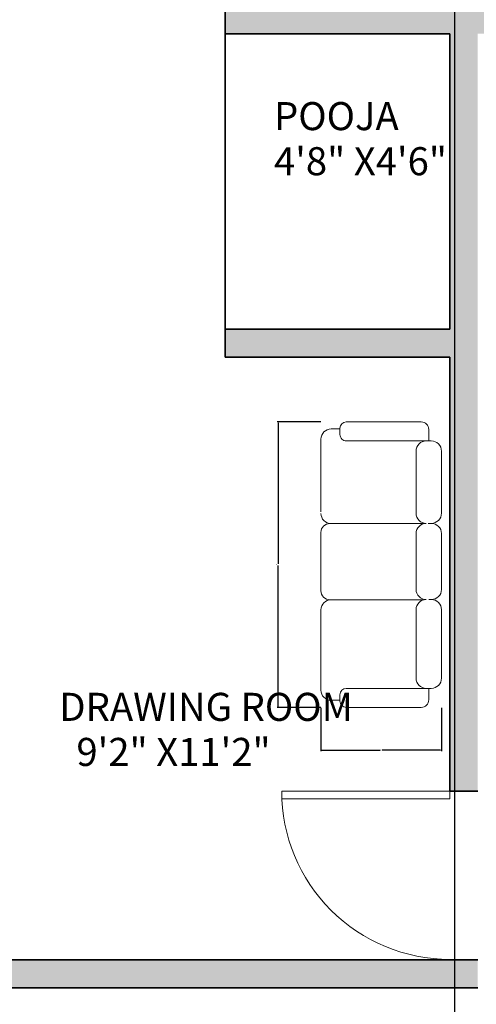
# Model space of a CAD drawing. Units: inches. Extents: x 2070 to 4408, y 1595 to 4269.
# Tile 6 of 20: x 2247 to 2345, y 1739 to 1949. Entities that reach past the tile are written whole.
import ezdxf

# ---------------------------------------------------------------- set-up
doc = ezdxf.new("R2010")
doc.units = ezdxf.units.IN
for name, color, linetype, lineweight in [('A-ANNO-DIMS', 2, 'Continuous', 18), ('A-AREA-IDEN', 7, 'Continuous', 18), ('A-DOOR', 4, 'Continuous', 18), ('A-FURN', 8, 'Continuous', 18), ('A-WALL', 7, 'Continuous', 35)]:
    doc.layers.add(name, color=color, linetype=linetype, lineweight=lineweight)
doc.layers.add('A-WALL-PATT', color=18, linetype='Continuous', lineweight=13, true_color=0x000000)
doc.styles.get("Standard").update_dxf_attribs({"font": 'arial.ttf'})
doc.dimstyles.get("Standard").update_dxf_attribs({"dimtxt": 0.18, "dimasz": 0.18, "dimexe": 0.18, "dimexo": 0.0625, "dimgap": 0.09, "dimtad": 0, "dimtih": 1, "dimtoh": 1, "dimdec": 4, "dimzin": 0, "dimdsep": 46, "dimtxsty": 'Standard', "dimcen": 0.09, "dimadec": 0, "dimazin": 0, "dimtfac": 1, "dimtdec": 4, "dimtofl": 0, "dimtmove": 0, "dimatfit": 3, "dimfxl": 1, "dimtolj": 1, "dimtzin": 0, "dimarcsym": 0})

# ---------------------------------------------------------------- blocks, each defined once
blk = doc.blocks.new('*U3')
for p, q in [((0, 0), (0, 6)), ((40, 0), (40, 6))]:
    blk.add_line(p, q)
blk.add_lwpolyline([(0, 0), (0, -40), (1.75, -40), (1.75, 0)], close=True)
blk.add_arc((0, 0), 40, 270, 0)
blk = doc.blocks.new('A$C0876780F')
for p, q in [((0.72, 0.95), (0.23, 0.95)), ((1.32, 0.95), (0.88, 0.95)), ((1.48, 0.95), (2.02, 0.95)), ((0.15, 0.87), (0.15, 0.8444)), ((0.15, 0.87), (0.15, 0.85)), ((0.8, 0.85), (0.8, 0.87)), ((0.8, 0.87), (0.8, 0.85)), ((0.8, 0.87), (0.8, 0.8444)), ((1.4, 0.85), (1.4, 0.87)), ((1.4, 0.85), (1.4, 0.87)), ((2.1, 0.87), (2.1, 0.85)), ((2.1, 0.87), (2.1, 0.8444)), ((0, 0.79), (0, 0.21)), ((0.15, 0.85), (0.06, 0.85)), ((0.15, 0.21), (0.15, 0.85)), ((0.8011, 0.8204), (0.8011, 0.08)), ((1.4014, 0.08), (1.4014, 0.803)), ((2.1, 0.21), (2.1, 0.85)), ((2.1, 0.85), (2.19, 0.85)), ((2.25, 0.79), (2.25, 0.21)), ((0.72, 0.75), (0.23, 0.75)), ((1.32, 0.75), (0.88, 0.75)), ((1.48, 0.75), (2.02, 0.75)), ((0.15, 0.2), (0.15, 0.25)), ((2.1, 0.2), (2.1, 0.25)), ((0, 0.21), (0, 0.2)), ((2.25, 0.21), (2.25, 0.2)), ((0.05, 0.15), (0.1, 0.15)), ((0.056, 0.15), (0.056, 0.08)), ((0.8011, 0.07), (0.8011, 0.08)), ((1.4014, 0.07), (1.4014, 0.08)), ((2.2, 0.15), (2.15, 0.15)), ((2.194, 0.15), (2.194, 0.08)), ((0.136, 0), (0.7093, 0)), ((0.8711, 0), (1.3314, 0)), ((2.114, 0), (1.48, 0))]:
    blk.add_line(p, q)
for centre, radius, start, end in [((0.23, 0.87), 0.08, 90, 180), ((0.72, 0.87), 0.08, 0, 90), ((0.88, 0.87), 0.08, 90, 180), ((1.32, 0.87), 0.08, 0, 90), ((1.48, 0.87), 0.08, 90, 180), ((2.02, 0.87), 0.08, 0, 90), ((0.06, 0.79), 0.06, 90, 180), ((0.23, 0.83), 0.08, 180, 270), ((0.23, 0.83), 0.08, 180, 270), ((0.72, 0.83), 0.08, 270, 0), ((0.88, 0.83), 0.08, 180, 270), ((0.88, 0.83), 0.08, 180, 270), ((1.32, 0.83), 0.08, 270, 0), ((1.48, 0.83), 0.08, 180, 270), ((2.02, 0.83), 0.08, 270, 0), ((2.02, 0.83), 0.08, 270, 0), ((2.19, 0.79), 0.06, 0, 90), ((0.05, 0.2), 0.05, 180, 270), ((0.1, 0.2), 0.05, 270, 0), ((0.09, 0.21), 0.06, 350.53768, 0), ((2.16, 0.21), 0.06, 180, 189.46232), ((2.15, 0.2), 0.05, 180, 270), ((2.2, 0.2), 0.05, 270, 0), ((0.136, 0.08), 0.08, 180, 270), ((0.7211, 0.08), 0.08, 270, 0), ((1.4814, 0.08), 0.08, 180, 270), ((2.114, 0.08), 0.08, 270, 0), ((0.8711, 0.07), 0.07, 180, 270), ((1.3314, 0.07), 0.07, 270, 0)]:
    blk.add_arc(centre, radius, start, end)
blk = doc.blocks.new('*D21')
at = {"layer": 'A-ANNO-DIMS', "color": 0, "lineweight": -2, "transparency": 16777216}
for p, q in [((2311.6, 1863.4), (2302.32, 1863.4)), ((2302.5, 1863.22), (2302.5, 1833.06)), ((2302.5, 1802.53), (2302.5, 1832.69)), ((2311.6, 1802.35), (2302.32, 1802.35))]:
    blk.add_line(p, q, dxfattribs=at)
at = {"layer": 'A-ANNO-DIMS', "color": 0, "transparency": 16777216}
for points in [[(2302.47, 1863.22), (2302.53, 1863.22), (2302.5, 1863.4)], [(2302.47, 1802.53), (2302.53, 1802.53), (2302.5, 1802.35)]]:
    blk.add_solid(points, dxfattribs=at)
at = {"layer": 'Defpoints', "color": 0, "transparency": 16777216}
for p in [(2311.66, 1863.4), (2302.5, 1802.35), (2311.66, 1802.35)]:
    blk.add_point(p, dxfattribs=at)
at = {"layer": 'A-ANNO-DIMS', "color": 0, "transparency": 16777216, "insert": (2302.5, 1832.87), "char_height": 0.18, "attachment_point": 5}
blk.add_mtext('\\A1;SOFA 61', dxfattribs=at)
blk = doc.blocks.new('*D22')
at = {"layer": 'A-ANNO-DIMS', "color": 0, "lineweight": -2, "transparency": 16777216}
for p, q in [((2311.66, 1802.28), (2311.66, 1793.01)), ((2337.44, 1802.28), (2337.44, 1793.01)), ((2311.84, 1793.19), (2324.33, 1793.19)), ((2337.26, 1793.19), (2324.77, 1793.19))]:
    blk.add_line(p, q, dxfattribs=at)
at = {"layer": 'A-ANNO-DIMS', "color": 0, "transparency": 16777216}
for points in [[(2311.84, 1793.22), (2311.84, 1793.16), (2311.66, 1793.19)], [(2337.26, 1793.22), (2337.26, 1793.16), (2337.44, 1793.19)]]:
    blk.add_solid(points, dxfattribs=at)
at = {"layer": 'Defpoints', "color": 0, "transparency": 16777216}
for p in [(2311.66, 1802.35), (2337.44, 1802.35), (2337.44, 1793.19)]:
    blk.add_point(p, dxfattribs=at)
at = {"layer": 'A-ANNO-DIMS', "color": 0, "transparency": 16777216, "insert": (2324.55, 1793.19), "char_height": 0.18, "attachment_point": 5}
blk.add_mtext('\\A1;26', dxfattribs=at)
blk = doc.blocks.new('*D24')
at = {"layer": 'A-ANNO-DIMS', "color": 0, "lineweight": -2, "transparency": 16777216}
for p, q in [((2103.13, 2291.4), (2069.84, 2291.4)), ((2070.02, 2291.22), (2070.02, 1960.08)), ((2070.02, 1628.58), (2070.02, 1959.72)), ((2336.13, 1628.4), (2069.84, 1628.4))]:
    blk.add_line(p, q, dxfattribs=at)
at = {"layer": 'A-ANNO-DIMS', "color": 0, "transparency": 16777216}
for points in [[(2069.99, 2291.22), (2070.05, 2291.22), (2070.02, 2291.4)], [(2069.99, 1628.58), (2070.05, 1628.58), (2070.02, 1628.4)]]:
    blk.add_solid(points, dxfattribs=at)
at = {"layer": 'Defpoints', "color": 0, "transparency": 16777216}
for p in [(2070.02, 2291.4), (2103.2, 2291.4), (2336.2, 1628.4)]:
    blk.add_point(p, dxfattribs=at)
at = {"layer": 'A-ANNO-DIMS', "color": 0, "transparency": 16777216, "insert": (2070.02, 1959.9), "char_height": 0.18, "attachment_point": 5}
blk.add_mtext('\\A1;663', dxfattribs=at)
blk = doc.blocks.new('*D32')
at = {"layer": 'A-ANNO-DIMS', "color": 0, "lineweight": -2, "transparency": 16777216}
for p, q in [((2245.2, 2230.58), (2245.2, 1595.04)), ((2340.2, 2230.58), (2340.2, 1595.04)), ((2245.38, 1595.22), (2292.48, 1595.22)), ((2340.02, 1595.22), (2292.92, 1595.22))]:
    blk.add_line(p, q, dxfattribs=at)
at = {"layer": 'A-ANNO-DIMS', "color": 0, "transparency": 16777216}
for points in [[(2245.38, 1595.25), (2245.38, 1595.19), (2245.2, 1595.22)], [(2340.02, 1595.25), (2340.02, 1595.19), (2340.2, 1595.22)]]:
    blk.add_solid(points, dxfattribs=at)
at = {"layer": 'Defpoints', "color": 0, "transparency": 16777216}
for p in [(2245.2, 2230.65), (2340.2, 2230.65), (2340.2, 1595.22)]:
    blk.add_point(p, dxfattribs=at)
at = {"layer": 'A-ANNO-DIMS', "color": 0, "transparency": 16777216, "insert": (2292.7, 1595.22), "char_height": 0.18, "attachment_point": 5}
blk.add_mtext('\\A1;95', dxfattribs=at)

msp = doc.modelspace()

# ---------------------------------------------------------------- hatches: boundary and pattern name
at = {"layer": 'A-WALL-PATT'}
h = msp.add_hatch(color=256, dxfattribs=at)
h.dxf.hatch_style = 1
h.paths.add_polyline_path([(2346.196, 2218.3995), (2346.196, 2282.3995), (2340.196, 2282.3995), (2340.196, 2212.3995), (2345.5866, 2212.3995), (2346.196, 2212.3995)], flags=0)
h.paths.add_polyline_path([(2245.196, 2282.3995), (2239.196, 2282.3995), (2239.196, 2186.3995), (2244.5866, 2186.3995), (2245.196, 2186.3995)], flags=0)
h.paths.add_polyline_path([(2340.196, 2230.6455), (2245.196, 2230.6455), (2245.196, 2224.6455), (2340.196, 2224.6455)], flags=0)
h.paths.add_polyline_path([(2245.196, 2150.3995), (2239.196, 2150.3995), (2164.4362, 2150.3995), (2164.4362, 2144.3995), (2239.196, 2144.3995), (2239.196, 2086.3995), (2239.196, 2067.2711), (2244.5866, 2067.2711), (2245.196, 2067.2711), (2245.196, 2144.3995)], flags=0)
h.paths.add_polyline_path([(2346.196, 2176.3995), (2340.196, 2176.3995), (2340.196, 2086.3995), (2346.196, 2086.3995), (2346.196, 2125.318)], flags=0)
h.paths.add_polyline_path([(2446.196, 2086.3995), (2346.196, 2086.3995), (2340.196, 2086.3995), (2340.196, 2080.3995), (2446.196, 2080.3995)], flags=0)
h.paths.add_polyline_path([(2455.196, 2291.3995), (2103.196, 2291.3995), (2103.196, 1699.3995), (2336.196, 1699.3995), (2336.196, 1628.3995), (2345.196, 1628.3995), (2446.196, 1628.3995), (2454.8846, 1628.3995), (2454.8846, 1699.3995)])
h.paths.add_polyline_path([(2446.196, 2282.3995), (2446.196, 2218.3995), (2446.196, 2212.3995), (2446.196, 2086.3995), (2446.196, 2080.3995), (2446.196, 1708.3995), (2446.196, 1637.3995), (2345.196, 1637.3995), (2345.196, 1699.3995), (2345.196, 1708.3995), (2336.196, 1708.3995), (2112.196, 1708.3995), (2112.196, 2282.3995), (2239.196, 2282.3995), (2245.196, 2282.3995), (2356.196, 2282.3995)], flags=16)
h.paths.add_polyline_path([(2245.196, 2150.3995), (2245.196, 2144.3995), (2245.196, 2067.2711), (2244.5866, 2067.2711), (2239.196, 2067.2711), (2239.196, 2065.6988), (2203.2929, 2065.6988, 0.40145271), (2239.196, 2031.3337), (2244.5866, 2031.3337), (2245.196, 2031.2711), (2245.196, 1924.1525), (2239.196, 1924.1525), (2239.196, 1922.5803), (2203.2929, 1922.5803, 0.40145271), (2239.196, 1888.2151), (2244.5866, 1888.2151), (2245.196, 1888.1525), (2245.196, 1748.3995), (2339.196, 1748.4621, -0.40145271), (2303.2929, 1782.8272), (2303.2585, 1782.8272), (2303.2585, 1784.3995), (2339.196, 1784.3995), (2339.196, 1877.2067), (2291.196, 1877.2067), (2291.196, 1883.2067), (2291.196, 1946.3995), (2291.196, 1952.3995), (2291.196, 2086.3995), (2297.196, 2086.3995), (2302.196, 2086.3995), (2302.196, 2081.0259), (2303.7633, 2081.0259), (2303.7633, 2080.3995), (2338.0148, 2080.3995, 0.00437129), (2338.0203, 2081.0259), (2338.0203, 2086.3995), (2340.196, 2086.3995), (2340.196, 2176.4621), (2345.5866, 2176.4621, 0.40145271), (2381.4896, 2210.8272), (2345.5866, 2210.8272), (2345.5866, 2212.3995), (2340.196, 2212.3995), (2340.196, 2224.6455), (2245.196, 2224.6455), (2245.196, 2186.3995), (2244.5866, 2186.3995), (2239.196, 2186.3995), (2239.196, 2184.8272), (2203.2929, 2184.8272, 0.40145271), (2239.196, 2150.4621), (2244.5866, 2150.4621)], flags=0)
h.paths.add_polyline_path([(2346.196, 2282.3995), (2346.196, 2218.3995), (2377.1813, 2218.3995), (2377.1813, 2212.3995), (2346.196, 2212.3995), (2345.5866, 2212.3995), (2340.196, 2212.3995), (2340.196, 2224.6455), (2245.196, 2224.6455), (2245.196, 2230.6455), (2245.196, 2282.3995), (2292.696, 2256.5225), (2340.196, 2282.3995)], flags=0)
h.paths.add_polyline_path([(2346.196, 2086.3995), (2340.196, 2086.3995), (2340.196, 2080.3995), (2446.196, 2080.3995), (2431.196, 2016.3995), (2446.196, 1952.3995), (2412.196, 1952.3995), (2412.196, 2080.3995), (2340.196, 2080.3995), (2340.196, 2086.3995), (2340.196, 2176.3995), (2346.196, 2176.3995), (2346.196, 2125.318)], flags=0)
h.paths.add_polyline_path([(2186.508, 2270.0471, -0.03755288), (2186.9712, 2269.8581), (2186.9164, 2270.112, -0.02759121)], flags=0)
h.paths.add_polyline_path([(2183.955, 2273.7766, 1), (2188.2945, 2273.7766, 1)], flags=0)
h.paths.add_polyline_path([(2142.5261, 2274.6158, -0.03707541), (2142.5672, 2275.1696), (2142.5672, 2276.826), (2119.8759, 2276.826), (2119.8759, 2263.0962), (2140.4332, 2263.0962), (2142.5672, 2263.0962), (2142.5672, 2274.0621, -0.03707541)], flags=0)
h.paths.add_polyline_path([(2209.8974, 2263.0962), (2209.8974, 2262.2079), (2190.8042, 2262.2079), (2190.8042, 2263.0962)], flags=0)
h.paths.add_polyline_path([(2210.6382, 2276.1833), (2210.6382, 2263.9844), (2190.2185, 2263.9844), (2190.2185, 2276.1833)], flags=0)
h.paths.add_polyline_path([(2188.4362, 2273.7766, -1), (2183.8133, 2273.7766, -1)], flags=0)
h.paths.add_polyline_path([(2245.196, 2150.3995), (2245.196, 2144.3995), (2245.196, 2067.2711), (2239.196, 2067.2711), (2239.196, 2080.3995), (2172.196, 2080.3995), (2172.196, 2000.3995), (2239.196, 2000.3995), (2239.196, 1940.3995), (2159.0187, 1940.3995), (2123.0187, 1940.3995), (2112.196, 1940.3995), (2112.196, 1946.3995), (2123.0187, 1946.3995), (2123.0187, 1982.2238), (2124.586, 1982.2238), (2124.586, 1982.1895, -0.40145271), (2158.8429, 1946.3995), (2159.0187, 1946.3995), (2239.196, 1946.3995), (2239.196, 1994.3995), (2112.196, 1994.3995), (2112.196, 2000.3995), (2139.196, 2040.3995), (2112.196, 2080.3995), (2112.196, 2086.3995), (2239.196, 2086.3995), (2239.196, 2144.3995), (2209.5809, 2144.3995), (2209.5809, 2136.3995), (2203.0809, 2136.3995), (2205.0809, 2130.3996, -0.70257121), (2199.081, 2116.3995, -0.70256205), (2193.0809, 2130.3994), (2195.0809, 2136.3995), (2192.0809, 2136.3995), (2192.0809, 2134.8995), (2189.0809, 2134.8995), (2189.0809, 2135.8995), (2191.0809, 2135.8995), (2191.0809, 2136.3995), (2188.5809, 2136.3995), (2188.5809, 2144.3995), (2164.2481, 2144.3995, -0.39385849), (2130.0035, 2109.5491), (2130.0035, 2109.5147), (2128.4362, 2109.5147), (2128.4362, 2144.3995), (2112.196, 2144.3995), (2112.196, 2150.3995), (2128.4362, 2150.3995), (2128.4362, 2150.7127), (2164.4362, 2150.7127), (2164.4362, 2150.3995), (2239.196, 2150.3995)], flags=0)
h.paths.add_polyline_path([(2188.2075, 2266.8735), (2188.2075, 2211.8632, -0.41421356), (2185.4833, 2209.1391), (2146.7995, 2209.1391, -0.41421356), (2144.0754, 2211.8632), (2144.0754, 2266.8735, -0.41421356), (2146.7995, 2269.5976), (2185.4833, 2269.5976, -0.41421356)], flags=0)
h.paths.add_polyline_path([(2185.0844, 2273.7766, -1), (2187.1651, 2273.7766, -1)], flags=0)
h.paths.add_polyline_path([(2182.0486, 2259.2932), (2168.0953, 2259.2932), (2168.0953, 2260.8424), (2163.7261, 2260.8424), (2163.7261, 2259.2932), (2149.7727, 2259.2932), (2149.7727, 2266.3352), (2163.7261, 2266.3352), (2163.7261, 2261.9839), (2168.0953, 2261.9839), (2168.0953, 2266.3352), (2182.0486, 2266.3352)], flags=0)
h.paths.add_polyline_path([(2148.2585, 2250.2051), (2153.0615, 2241.8861, 0.39807048)], flags=0)
h.paths.add_polyline_path([(2162.7572, 2247.2885), (2153.1461, 2241.7396), (2148.1083, 2250.4653), (2157.7194, 2256.0142)], flags=0)
h.paths.add_polyline_path([(2162.6726, 2247.4351, -0.39286196), (2157.8415, 2255.6313), (2157.6431, 2255.6313), (2157.8696, 2255.7541)], flags=0)
h.paths.add_polyline_path([(2164.2604, 2145.339), (2164.4362, 2144.3995), (2164.4362, 2150.3995), (2164.2604, 2150.7127)], flags=0)
h.paths.add_polyline_path([(2208.5809, 2142.6495), (2208.5809, 2138.3995, -0.41421356), (2207.8309, 2137.3995), (2190.5809, 2137.3995, -0.41421356), (2189.5809, 2138.1495), (2189.5809, 2142.3995, -0.41421356), (2190.3309, 2143.3995), (2207.5809, 2143.3995, -0.41421356)], flags=0)
h.paths.add_polyline_path([(2147.957, 2229.9119), (2154.7494, 2223.1195, 0.39807048)], flags=0)
h.paths.add_polyline_path([(2162.7165, 2230.8473), (2154.8691, 2222.9998), (2147.7446, 2230.1244), (2155.592, 2237.9718)], flags=0)
h.paths.add_polyline_path([(2162.5969, 2230.9669, -0.39807048), (2155.8044, 2237.7594)], flags=0)
h.paths.add_polyline_path([(2391.8776, 2049.9192), (2408.5766, 2049.9192), (2408.5766, 2033.2202), (2408.5766, 1983.123), (2408.5766, 1966.4239), (2391.8776, 1966.4239), (2391.8776, 1983.123), (2341.7804, 1983.123), (2341.7804, 2033.2202), (2391.8776, 2033.2202)], flags=0)
h.paths.add_polyline_path([(2144.1055, 2274.6158, 1), (2148.445, 2274.6158, 1)], flags=0)
h.paths.add_polyline_path([(2148.5867, 2274.6158, -1), (2143.9638, 2274.6158, -1)], flags=0)
h.paths.add_polyline_path([(2145.2349, 2274.6158, -1), (2147.3156, 2274.6158, -1)], flags=0)
edge = h.paths.add_edge_path(flags=0)
edge.add_ellipse((2400.5951, 2040.9436), major_axis=(-4.5109, 0), ratio=0.97544784, start_angle=180, end_angle=270, ccw=False)
edge.add_ellipse((2400.5951, 2040.9436), major_axis=(-4.5109, 0), ratio=0.97544784, start_angle=90, end_angle=180, ccw=False)
edge.add_ellipse((2400.5951, 2040.9436), major_axis=(-4.5109, 0), ratio=0.97544784, start_angle=0, end_angle=90, ccw=False)
edge.add_ellipse((2400.5951, 2040.9436), major_axis=(-4.5109, 0), ratio=0.97544784, start_angle=270, end_angle=360, ccw=False)
h.paths.add_polyline_path([(2199.0809, 2117.3995, -0.73452973), (2195.0809, 2130.3995), (2203.081, 2130.3995, -0.73453329)], flags=0)
h.paths.add_polyline_path([(2141.9147, 2276.0353), (2141.9147, 2263.9844), (2120.4685, 2263.9844), (2120.4685, 2276.0353)], flags=0)
h.paths.add_polyline_path([(2138.4481, 2273.4072), (2138.4481, 2266.7226), (2133.2801, 2266.7226), (2133.2801, 2273.4072)], flags=0)
h.paths.add_polyline_path([(2137.9691, 2272.9175), (2137.9691, 2272.204), (2135.4229, 2272.204), (2135.4229, 2271.6329), (2135.3221, 2270.1051), (2135.3221, 2269.0265), (2135.4229, 2268.6811), (2135.4229, 2267.2011), (2133.7212, 2267.2011), (2133.7212, 2268.6811), (2133.7983, 2269.9587), (2133.7983, 2271.2758), (2133.7212, 2271.6329), (2133.7212, 2273.0065), (2135.717, 2273.0065), (2135.717, 2272.9175)], flags=0)
h.paths.add_polyline_path([(2137.9215, 2271.8264), (2137.9215, 2271.3786), (2137.5182, 2271.3786), (2136.9355, 2271.3786), (2136.3529, 2271.3786), (2135.7703, 2271.3786), (2135.7703, 2271.8264), (2136.1736, 2271.8264), (2136.7562, 2271.8264), (2137.3389, 2271.8264)], flags=0)
h.paths.add_polyline_path([(2137.9215, 2271.692), (2137.5182, 2271.692), (2136.9355, 2271.513), (2137.3389, 2271.513)], flags=0)
h.paths.add_polyline_path([(2136.3529, 2271.692), (2135.7703, 2271.513), (2136.1736, 2271.513), (2136.7562, 2271.692)], flags=0)
h.paths.add_polyline_path([(2137.9215, 2271.513), (2137.5182, 2271.513), (2136.7562, 2271.747), (2136.7562, 2271.692), (2137.3389, 2271.692)], flags=0)
h.paths.add_polyline_path([(2137.8207, 2270.4664), (2137.8207, 2270.0971), (2137.8207, 2269.627), (2137.8207, 2269.1569), (2137.8207, 2268.6868), (2137.3837, 2268.6868), (2136.6442, 2268.6868), (2135.9271, 2268.6868), (2135.9271, 2269.0562), (2135.9271, 2269.5263), (2135.9271, 2269.9963), (2135.9271, 2270.4664), (2136.3641, 2270.4664), (2137.0812, 2270.4664)], flags=0)
h.paths.add_polyline_path([(2137.3837, 2269.627), (2137.8207, 2269.627), (2137.8207, 2269.5263), (2137.3837, 2269.5263), (2137.3837, 2269.1569), (2137.8207, 2269.1569), (2137.3837, 2269.0562), (2137.3837, 2268.6868), (2137.0812, 2268.6868), (2137.0812, 2269.0562), (2136.6442, 2269.0562), (2136.6442, 2268.6868), (2136.3641, 2268.6868), (2136.3641, 2269.0562), (2135.9271, 2269.0562), (2135.9271, 2269.1569), (2136.3641, 2269.1569), (2136.3641, 2269.5263), (2135.9271, 2269.5263), (2135.9271, 2269.627), (2136.3641, 2269.627), (2136.3641, 2269.9963), (2135.9271, 2269.9963), (2136.3641, 2270.0971), (2136.3641, 2270.4664), (2136.6442, 2270.4664), (2136.6442, 2270.0971), (2137.0812, 2270.0971), (2137.0812, 2270.4664), (2137.3837, 2270.4664), (2137.3837, 2270.0971), (2137.8207, 2270.0971), (2137.3837, 2269.9963)], flags=0)
h.paths.add_polyline_path([(2137.5182, 2271.8264), (2137.5182, 2271.692), (2137.3389, 2271.3786), (2137.3389, 2271.513)], flags=0)
h.paths.add_polyline_path([(2137.8179, 2267.8138), (2137.8179, 2267.6879), (2137.1876, 2267.6879), (2136.4733, 2267.6879), (2135.759, 2267.6879), (2135.759, 2267.8138), (2136.3893, 2267.8138), (2137.1036, 2267.8138)], flags=0)
h.paths.add_polyline_path([(2137.0812, 2269.9963), (2137.0812, 2269.627), (2137.0812, 2269.1569), (2136.6442, 2269.1569), (2136.6442, 2269.5263), (2136.6442, 2269.9963)], flags=0)
h.paths.add_polyline_path([(2136.3529, 2271.8264), (2136.3529, 2271.692), (2136.1736, 2271.3786), (2136.1736, 2271.513)], flags=0)
h.paths.add_polyline_path([(2136.4733, 2267.8138), (2136.4733, 2267.6879), (2136.3893, 2267.6879), (2136.3893, 2267.8138)], flags=0)
h.paths.add_polyline_path([(2407.9087, 2032.5522), (2407.9087, 1983.7909), (2359.81, 1983.7909, -0.00912788), (2359.0575, 1983.7909), (2342.4483, 1983.7909), (2342.4483, 2032.5522)], flags=0)
h.paths.add_polyline_path([(2389.1838, 2023.1358), (2353.7856, 2023.1358), (2353.7856, 1985.4867, -0.09210376), (2350.2788, 1988.655), (2350.2788, 2026.6426), (2389.1838, 2026.6426)], flags=0)
h.paths.add_polyline_path([(2352.6166, 2024.3048), (2351.4477, 2024.3048), (2351.4477, 2025.4737), (2352.6166, 2025.4737)], flags=0)
h.paths.add_polyline_path([(2399.6319, 2026.7589), (2404.3661, 2026.7589, -0.41421356), (2407.0379, 2024.087), (2407.0379, 2013.4908, -0.41421356), (2404.3661, 2010.819), (2399.6319, 2010.819, -0.41421356), (2396.96, 2013.4908), (2396.96, 2024.087, -0.41421356)], flags=0)
h.paths.add_polyline_path([(2399.6319, 2026.0909), (2404.3661, 2026.0909, -0.41421356), (2406.37, 2024.087), (2406.37, 2013.4908, -0.41421356), (2404.3661, 2011.487), (2399.6319, 2011.487, -0.41421356), (2397.628, 2013.4908), (2397.628, 2024.087, -0.41421356)], flags=0)
h.paths.add_polyline_path([(2399.6319, 2002.3217), (2404.3661, 2002.3217, -0.41421356), (2407.0379, 1999.6498), (2407.0379, 1989.0536, -0.41421356), (2404.3661, 1986.3818), (2399.6319, 1986.3818, -0.41421356), (2396.96, 1989.0536), (2396.96, 1999.6498, -0.41421356)], flags=0)
h.paths.add_polyline_path([(2399.6319, 2001.6537), (2404.3661, 2001.6537, -0.41421356), (2406.37, 1999.6498), (2406.37, 1989.0536, -0.41421356), (2404.3661, 1987.0497), (2399.6319, 1987.0497, -0.41421356), (2397.628, 1989.0536), (2397.628, 1999.6498, -0.41421356)], flags=0)
edge = h.paths.add_edge_path(flags=0)
edge.add_ellipse((2400.5951, 1975.3996), major_axis=(-4.5109, 0), ratio=0.97544784, start_angle=-180, end_angle=-90, ccw=False)
edge.add_ellipse((2400.5951, 1975.3996), major_axis=(-4.5109, 0), ratio=0.97544784, start_angle=90, end_angle=180, ccw=False)
edge.add_ellipse((2400.5951, 1975.3996), major_axis=(-4.5109, 0), ratio=0.97544784, start_angle=0, end_angle=90, ccw=False)
edge.add_ellipse((2400.5951, 1975.3996), major_axis=(-4.5109, 0), ratio=0.97544784, start_angle=-90, end_angle=0, ccw=False)
h.paths.add_polyline_path([(2345.196, 1910.3995), (2366.4386, 1910.3995), (2366.4386, 1925.4555), (2392.3856, 1925.4555), (2392.3856, 1933.5025), (2400.1399, 1925.4555), (2392.3856, 1919.8795), (2392.3856, 1925.4555), (2366.4386, 1925.4555), (2366.4386, 1910.3995), (2381.196, 1910.3995), (2405.196, 1910.3995), (2405.196, 1898.3995), (2446.196, 1898.3995), (2446.196, 1886.3995), (2405.196, 1886.3995), (2405.196, 1874.3995), (2446.196, 1874.3995), (2446.196, 1862.3995), (2405.196, 1862.3995), (2405.196, 1850.3995), (2446.196, 1850.3995), (2446.196, 1838.3995), (2405.196, 1838.3995), (2405.196, 1826.3995), (2446.196, 1826.3995), (2446.196, 1814.3995), (2405.196, 1814.3995), (2405.196, 1802.3995), (2446.196, 1802.3995), (2446.196, 1798.3995), (2446.196, 1792.3995), (2405.196, 1792.3995), (2405.196, 1910.3995), (2381.196, 1910.3995), (2381.196, 1792.3995), (2345.196, 1792.3995)], flags=0)
h.paths.add_polyline_path([(2333.0944, 1863.3993, -0.41421356), (2334.7225, 1861.7712), (2334.7225, 1859.329), (2335.2653, 1859.329, -0.41421356), (2337.4361, 1857.1582), (2337.4361, 1843.862, -0.41421356), (2335.2653, 1841.6911, -0.41421356), (2337.4361, 1839.5203), (2337.4361, 1827.5808, -0.41421356), (2335.2653, 1825.41, -0.41421356), (2337.4361, 1823.2392), (2337.4361, 1808.5862, -0.41421356), (2335.2653, 1806.4153), (2334.7225, 1806.4153), (2334.7225, 1803.9732, -0.41421356), (2333.0944, 1802.3451), (2317.356, 1802.3451), (2317.0846, 1802.3451, -0.41421356), (2315.7279, 1803.7018), (2315.7279, 1803.8646), (2313.8284, 1803.8646, -0.41421356), (2311.6576, 1806.0354), (2311.6576, 1823.2015, -0.39597602), (2313.6834, 1825.3765, -0.43384798), (2311.6576, 1827.2718), (2311.6576, 1839.761, -0.41421356), (2313.5571, 1841.6604), (2313.8284, 1841.6604), (2333.8159, 1841.6604, -0.04213623), (2334.1798, 1841.6911, -0.41421356), (2332.009, 1843.862), (2332.009, 1857.1582, -0.41421356), (2334.1798, 1859.329), (2317.356, 1859.329), (2317.0846, 1859.329, -0.41421356), (2315.7279, 1860.6858), (2315.7279, 1862.0426, -0.41421356), (2317.0846, 1863.3993), (2317.356, 1863.3993)], flags=0)
h.paths.add_polyline_path([(2208.8475, 1848.9818), (2208.8475, 1840.9741, -0.41421356), (2207.0458, 1839.1724), (2206.5453, 1839.1721), (2206.5453, 1838.7218, -0.40985861), (2204.7704, 1836.9203), (2183.7501, 1836.9203, -0.41858196), (2181.9216, 1838.7218), (2181.9216, 1839.1721), (2181.421, 1839.1724, -0.41421356), (2179.6193, 1840.9741), (2179.6193, 1848.6817, -0.44064415), (2185.1126, 1854.9874), (2203.3852, 1854.9874, -0.45707961)], flags=0)
h.paths.add_polyline_path([(2204.243, 1848.4815), (2204.243, 1848.4815, 0.41725335), (2202.2204, 1850.4833), (2186.2049, 1850.4833, 0.4111805), (2184.2237, 1848.4815), (2184.2237, 1848.4815, -0.4111807), (2186.2049, 1850.4833), (2202.2204, 1850.4833, -0.41725315)], flags=0)
h.paths.add_polyline_path([(2234.7177, 1830.228), (2234.7176, 1781.6047, -0.41421356), (2233.4381, 1780.3252), (2218.6064, 1780.3252, -0.41421356), (2217.8387, 1781.0929), (2217.8387, 1783.3961, -0.41421356), (2218.6064, 1784.1639), (2218.6065, 1796.9595, -0.41421356), (2219.886, 1798.239, -0.41421356), (2218.6065, 1799.5186), (2218.6065, 1812.3142, -0.41421356), (2219.8861, 1813.5938, -0.41421356), (2218.6065, 1814.8733), (2218.6065, 1827.6689, -0.41421356), (2217.8388, 1828.4367), (2217.8388, 1830.7399, -0.41421356), (2218.6065, 1831.5076), (2233.4382, 1831.5076, -0.41421356)], flags=0)
h.paths.add_polyline_path([(2230.6344, 1827.6689, -0.41421356), (2231.4021, 1826.9012), (2231.4021, 1784.9316, -0.41421356), (2230.6343, 1784.1639), (2221.1853, 1784.1639), (2221.1853, 1827.6689)], flags=0)
h.paths.add_polyline_path([(2222.7208, 1798.239), (2221.6971, 1798.239), (2221.6971, 1813.5938), (2222.7208, 1813.5938)], flags=0)
h.paths.add_polyline_path([(2206.5453, 1773.935), (2206.5453, 1773.4848), (2206.9457, 1773.4848), (2207.0458, 1773.4845, -0.41421356), (2208.8475, 1771.6827), (2208.8475, 1763.675, -0.44222432), (2203.6505, 1757.6695), (2185.3851, 1757.6695, -0.45508402), (2179.6193, 1763.9752), (2179.6193, 1771.6827, -0.41421356), (2181.421, 1773.4845), (2181.421, 1773.4848), (2181.9216, 1773.4848), (2181.9216, 1773.935, -0.40985861), (2183.6965, 1775.7366), (2204.7167, 1775.7366, -0.41858196)], flags=0)
h.paths.add_polyline_path([(2202.2619, 1762.1736), (2186.2464, 1762.1736, -0.41725315), (2184.2237, 1764.1754), (2184.2237, 1764.1754, 0.41725335), (2186.2464, 1762.1736), (2202.2619, 1762.1736, 0.4111805), (2204.243, 1764.1754), (2204.243, 1764.1754, -0.4111807)], flags=0)
h.paths.add_polyline_path([(2313.0034, 1713.1906), (2312.997, 1713.1697), (2313.0123, 1713.1612)], flags=0)
h.paths.add_polyline_path([(2305.7314, 1721.0488), (2305.6257, 1721.1994), (2305.4853, 1721.084)], flags=0)
h.paths.add_polyline_path([(2307.5562, 1726.1427), (2307.6186, 1726.1026), (2307.5737, 1726.0477), (2308.5692, 1720.6434), (2310.5345, 1721.2985), (2310.5721, 1721.411), (2310.6958, 1721.3523), (2313.8453, 1722.4021), (2314.9351, 1723.8033), (2314.9294, 1723.9165), (2315.0028, 1723.8903), (2313.874, 1722.4389), (2313.8697, 1722.4102), (2308.5692, 1720.6434), (2308.9864, 1720.122), (2309.0665, 1720.0971), (2309.053, 1720.0387), (2310.9235, 1717.7005), (2311.4182, 1717.6259), (2311.2918, 1717.2402), (2312.0655, 1716.2731), (2312.1081, 1716.2606), (2312.0969, 1716.2339), (2308.5692, 1720.6434), (2305.2249, 1717.745), (2305.232, 1717.704), (2305.1665, 1717.6944), (2308.5692, 1720.6434)], flags=0)
h.paths.add_polyline_path([(2288.2072, 1714.3431), (2288.2008, 1714.3222), (2288.216, 1714.3137)], flags=0)
h.paths.add_polyline_path([(2280.9352, 1722.2013), (2280.8295, 1722.3519), (2280.689, 1722.2365)], flags=0)
h.paths.add_polyline_path([(2282.76, 1727.2952), (2282.8224, 1727.2551), (2282.7775, 1727.2002), (2283.773, 1721.7959), (2285.7383, 1722.451), (2285.7759, 1722.5635), (2285.8995, 1722.5048), (2289.0491, 1723.5546), (2290.1389, 1724.9558), (2290.1332, 1725.069), (2290.2065, 1725.0428), (2289.0777, 1723.5915), (2289.0735, 1723.5628), (2283.773, 1721.7959), (2284.1901, 1721.2745), (2284.2703, 1721.2496), (2284.2567, 1721.1913), (2286.1273, 1718.8531), (2286.622, 1718.7785), (2286.4956, 1718.3927), (2287.2692, 1717.4256), (2287.3119, 1717.4131), (2287.3006, 1717.3864), (2283.773, 1721.7959), (2280.4286, 1718.8975), (2280.4357, 1718.8565), (2280.3703, 1718.8469), (2283.773, 1721.7959)], flags=0)
h.paths.add_polyline_path([(2302.0672, 1721.8694), (2301.8205, 1721.8572), (2301.7578, 1722.1787), (2299.415, 1724.5215), (2299.103, 1724.4694), (2299.0662, 1724.8703)], flags=0)
h.paths.add_polyline_path([(2264.5643, 1715.4956), (2264.5579, 1715.4747), (2264.5731, 1715.4662)], flags=0)
h.paths.add_polyline_path([(2257.2923, 1723.3538), (2257.1865, 1723.5044), (2257.0461, 1723.389)], flags=0)
h.paths.add_polyline_path([(2259.117, 1728.4477), (2259.1795, 1728.4077), (2259.1345, 1728.3527), (2260.13, 1722.9484), (2262.0954, 1723.6036), (2262.133, 1723.716), (2262.2566, 1723.6573), (2265.4061, 1724.7071), (2266.4959, 1726.1083), (2266.4902, 1726.2215), (2266.5636, 1726.1953), (2265.4348, 1724.744), (2265.4305, 1724.7153), (2260.13, 1722.9484), (2260.5472, 1722.427), (2260.6273, 1722.4022), (2260.6138, 1722.3438), (2262.4843, 1720.0056), (2262.979, 1719.931), (2262.8526, 1719.5452), (2263.6263, 1718.5781), (2263.6689, 1718.5656), (2263.6577, 1718.5389), (2260.13, 1722.9484), (2256.7857, 1720.05), (2256.7928, 1720.009), (2256.7273, 1719.9994), (2260.13, 1722.9484)], flags=0)
h.paths.add_polyline_path([(2277.2709, 1723.0219), (2277.0243, 1723.0097), (2276.9616, 1723.3312), (2274.6187, 1725.6741), (2274.3067, 1725.6219), (2274.27, 1726.0228)], flags=0)
h.paths.add_polyline_path([(2253.628, 1724.1744), (2253.3814, 1724.1622), (2253.3186, 1724.4838), (2250.9758, 1726.8266), (2250.6638, 1726.7744), (2250.627, 1727.1753)], flags=0)
h.paths.add_polyline_path([(2161.9194, 1715.4956), (2161.913, 1715.4747), (2161.9282, 1715.4662)], flags=0)
h.paths.add_polyline_path([(2154.6474, 1723.3538), (2154.5416, 1723.5044), (2154.4012, 1723.389)], flags=0)
h.paths.add_polyline_path([(2162.7899, 1724.744), (2162.7856, 1724.7153), (2157.4851, 1722.9484), (2157.9023, 1722.427), (2157.9824, 1722.4022), (2157.9689, 1722.3438), (2159.8394, 1720.0056), (2160.3341, 1719.931), (2160.2078, 1719.5452), (2160.9814, 1718.5781), (2161.024, 1718.5656), (2161.0128, 1718.5389), (2157.4851, 1722.9484), (2154.1408, 1720.05), (2154.1479, 1720.009), (2154.0824, 1719.9994), (2157.4851, 1722.9484), (2156.4721, 1728.4477), (2156.5346, 1728.4077), (2156.4896, 1728.3527), (2157.4851, 1722.9484), (2159.4505, 1723.6036), (2159.4881, 1723.716), (2159.6117, 1723.6573), (2162.7612, 1724.7071), (2163.851, 1726.1083), (2163.8453, 1726.2215), (2163.9187, 1726.1953)], flags=0)
h.paths.add_polyline_path([(2150.9831, 1724.1744), (2150.7365, 1724.1622), (2150.6738, 1724.4838), (2148.3309, 1726.8266), (2148.0189, 1726.7744), (2147.9822, 1727.1753)], flags=0)
h.paths.add_polyline_path([(2132.5099, 1716.6482), (2132.5035, 1716.6272), (2132.5187, 1716.6187)], flags=0)
h.paths.add_polyline_path([(2125.2379, 1724.5064), (2125.1322, 1724.6569), (2124.9917, 1724.5415)], flags=0)
h.paths.add_polyline_path([(2133.3804, 1725.8965), (2133.3762, 1725.8678), (2128.0757, 1724.101), (2128.4928, 1723.5795), (2128.5729, 1723.5547), (2128.5594, 1723.4963), (2130.43, 1721.1581), (2130.9246, 1721.0835), (2130.7983, 1720.6977), (2131.5719, 1719.7306), (2131.6146, 1719.7181), (2131.6033, 1719.6914), (2128.0757, 1724.101), (2124.7313, 1721.2025), (2124.7384, 1721.1615), (2124.6729, 1721.1519), (2128.0757, 1724.101), (2127.0626, 1729.6002), (2127.1251, 1729.5602), (2127.0801, 1729.5052), (2128.0757, 1724.101), (2130.041, 1724.7561), (2130.0786, 1724.8685), (2130.2022, 1724.8098), (2133.3517, 1725.8597), (2134.4415, 1727.2608), (2134.4358, 1727.3741), (2134.5092, 1727.3478)], flags=0)
h.paths.add_polyline_path([(2121.5736, 1725.3269), (2121.327, 1725.3148), (2121.2643, 1725.6363), (2118.9214, 1727.9791), (2118.6094, 1727.9269), (2118.5727, 1728.3279)], flags=0)
h.paths.add_polyline_path([(2433.3904, 1646.406), (2433.384, 1646.3851), (2433.3992, 1646.3766)], flags=0)
h.paths.add_polyline_path([(2426.1184, 1654.2642), (2426.0127, 1654.4148), (2425.8722, 1654.2994)], flags=0)
h.paths.add_polyline_path([(2427.9432, 1659.3581), (2428.0056, 1659.318), (2427.9606, 1659.2631), (2428.9562, 1653.8588), (2430.9215, 1654.514), (2430.9591, 1654.6264), (2431.0827, 1654.5677), (2434.2323, 1655.6175), (2435.322, 1657.0187), (2435.3163, 1657.1319), (2435.3897, 1657.1057), (2434.2609, 1655.6544), (2434.2567, 1655.6257), (2428.9562, 1653.8588), (2429.3733, 1653.3374), (2429.4534, 1653.3126), (2429.4399, 1653.2542), (2431.3105, 1650.916), (2431.8051, 1650.8414), (2431.6788, 1650.4556), (2432.4524, 1649.4885), (2432.4951, 1649.476), (2432.4838, 1649.4493), (2428.9562, 1653.8588), (2425.6118, 1650.9604), (2425.6189, 1650.9194), (2425.5535, 1650.9098), (2428.9562, 1653.8588)], flags=0)
h.paths.add_polyline_path([(2376.63, 1645.4912), (2376.6236, 1645.4703), (2376.6388, 1645.4617)], flags=0)
h.paths.add_polyline_path([(2369.358, 1653.3494), (2369.2523, 1653.5), (2369.1118, 1653.3845)], flags=0)
h.paths.add_polyline_path([(2371.1828, 1658.4432), (2371.2452, 1658.4032), (2371.2003, 1658.3482), (2372.1958, 1652.944), (2374.1611, 1653.5991), (2374.1987, 1653.7116), (2374.3224, 1653.6528), (2377.4719, 1654.7027), (2378.5617, 1656.1038), (2378.556, 1656.2171), (2378.6293, 1656.1908), (2377.5005, 1654.7395), (2377.4963, 1654.7108), (2372.1958, 1652.944), (2372.6129, 1652.4225), (2372.6931, 1652.3977), (2372.6795, 1652.3393), (2374.5501, 1650.0011), (2375.0448, 1649.9265), (2374.9184, 1649.5407), (2375.692, 1648.5737), (2375.7347, 1648.5611), (2375.7234, 1648.5344), (2372.1958, 1652.944), (2368.8514, 1650.0456), (2368.8586, 1650.0046), (2368.7931, 1649.995), (2372.1958, 1652.944)], flags=0)
h.paths.add_polyline_path([(2404.0947, 1645.0338), (2404.0883, 1645.0128), (2404.1035, 1645.0043)], flags=0)
h.paths.add_polyline_path([(2396.8227, 1652.892), (2396.717, 1653.0425), (2396.5765, 1652.9271)], flags=0)
h.paths.add_polyline_path([(2398.6475, 1657.9858), (2398.7099, 1657.9458), (2398.665, 1657.8908), (2399.6605, 1652.4866), (2401.6258, 1653.1417), (2401.6634, 1653.2541), (2401.7871, 1653.1954), (2404.9366, 1654.2453), (2406.0264, 1655.6464), (2406.0207, 1655.7596), (2406.094, 1655.7334), (2404.9652, 1654.2821), (2404.961, 1654.2534), (2399.6605, 1652.4866), (2400.0776, 1651.9651), (2400.1578, 1651.9403), (2400.1442, 1651.8819), (2402.0148, 1649.5437), (2402.5095, 1649.4691), (2402.3831, 1649.0833), (2403.1567, 1648.1162), (2403.1994, 1648.1037), (2403.1881, 1648.077), (2399.6605, 1652.4866), (2396.3162, 1649.5881), (2396.3233, 1649.5471), (2396.2578, 1649.5375), (2399.6605, 1652.4866)], flags=0)
h.paths.add_polyline_path([(2419.4532, 1658.0857), (2422.4541, 1655.0848), (2422.2075, 1655.0726), (2422.1448, 1655.3941), (2419.8019, 1657.737), (2419.4899, 1657.6848)], flags=0)
h.paths.add_polyline_path([(2390.1575, 1656.7135), (2393.1584, 1653.7125), (2392.9118, 1653.7004), (2392.8491, 1654.0219), (2390.5063, 1656.3647), (2390.1943, 1656.3125)], flags=0)
h.paths.add_polyline_path([(2362.6928, 1657.1709), (2365.6937, 1654.1699), (2365.4471, 1654.1578), (2365.3844, 1654.4793), (2363.0416, 1656.8221), (2362.7295, 1656.77)], flags=0)
h.paths.add_polyline_path([(2419.9523, 2037.8601), (2440.2872, 2037.8601), (2440.2872, 2047.1732), (2419.9523, 2047.1732)], flags=8)
h.paths.add_polyline_path([(2370.186, 1698.9005), (2413.6287, 1698.9005), (2413.6287, 1708.0908), (2370.186, 1708.0908)], flags=8)
h.paths.add_polyline_path([(2370.1656, 1708.5185), (2430.0857, 1708.5185), (2430.0857, 1717.8316), (2370.1656, 1717.8316)], flags=8)
h.paths.add_polyline_path([(2254.1469, 1788.1883), (2302.2471, 1788.1883), (2302.2471, 1797.3786), (2254.1469, 1797.3786)], flags=8)
h.paths.add_polyline_path([(2254.1264, 1797.8063), (2326.1448, 1797.8063), (2326.1448, 1807.1194), (2254.1264, 1807.1194)], flags=8)
h.paths.add_polyline_path([(2300.08, 1914.5069), (2338.861, 1914.5069), (2338.861, 1923.6972), (2300.08, 1923.6972)], flags=8)
h.paths.add_polyline_path([(2300.0595, 1924.1249), (2331.5882, 1924.1249), (2331.5882, 1933.438), (2300.0595, 1933.438)], flags=8)
h.paths.add_polyline_path([(2176.6905, 1716.4567), (2224.1441, 1716.4567), (2224.1441, 1725.647), (2176.6905, 1725.647)], flags=8)
h.paths.add_polyline_path([(2176.67, 1726.0747), (2245.9176, 1726.0747), (2245.9176, 1735.3878), (2176.67, 1735.3878)], flags=8)
h.paths.add_polyline_path([(2339.997, 2039.7696), (2388.1034, 2039.7696), (2388.1034, 2048.9661), (2339.997, 2048.9661)], flags=8)
h.paths.add_polyline_path([(2339.9776, 2049.3928), (2388.7204, 2049.3928), (2388.7204, 2058.7059), (2339.9776, 2058.7059)], flags=8)
h.paths.add_polyline_path([(2366.0063, 2161.3825), (2409.449, 2161.3825), (2409.449, 2170.5728), (2366.0063, 2170.5728)], flags=8)
h.paths.add_polyline_path([(2365.9868, 2171.0016), (2405.879, 2171.0016), (2405.879, 2180.3085), (2365.9868, 2180.3085)], flags=8)
h.paths.add_polyline_path([(2366.0102, 2247.0726), (2407.12, 2247.0726), (2407.12, 2256.263), (2366.0102, 2256.263)], flags=8)
h.paths.add_polyline_path([(2365.9897, 2256.6906), (2397.9686, 2256.6906), (2397.9686, 2266.0037), (2365.9897, 2266.0037)], flags=8)
h.paths.add_polyline_path([(2271.8465, 2102.7885), (2307.6541, 2102.7885), (2307.6541, 2111.9849), (2271.8465, 2111.9849)], flags=8)
h.paths.add_polyline_path([(2271.8281, 2112.4126), (2304.2673, 2112.4126), (2304.2673, 2121.7196), (2271.8281, 2121.7196)], flags=8)
h.paths.add_polyline_path([(2141.6408, 2187.5934), (2182.108, 2187.5934), (2182.108, 2196.7837), (2141.6408, 2196.7837)], flags=8)
h.paths.add_polyline_path([(2141.6203, 2197.2114), (2190.3631, 2197.2114), (2190.3631, 2206.5245), (2141.6203, 2206.5245)], flags=8)
h.paths.add_polyline_path([(2165.7271, 2103.039), (2211.5027, 2103.039), (2211.5027, 2112.2293), (2165.7271, 2112.2293)], flags=8)
h.paths.add_polyline_path([(2165.7077, 2112.658), (2185.1033, 2112.658), (2185.1033, 2121.965), (2165.7077, 2121.965)], flags=8)
h.paths.add_polyline_path([(2174.945, 2048.0789), (2211.3973, 2048.0789), (2211.3973, 2057.2693), (2174.945, 2057.2693)], flags=8)
h.paths.add_polyline_path([(2174.9256, 2057.698), (2194.3212, 2057.698), (2194.3212, 2067.0049), (2174.9256, 2067.0049)], flags=8)
h.paths.add_polyline_path([(2164.8305, 1965.8394), (2202.9649, 1965.8394), (2202.9649, 1975.0297), (2164.8305, 1975.0297)], flags=8)
h.paths.add_polyline_path([(2164.8111, 1975.4584), (2184.2067, 1975.4584), (2184.2067, 1984.7654), (2164.8111, 1984.7654)], flags=8)
h.paths.add_polyline_path([(2133.0392, 1862.086), (2173.5065, 1862.086), (2173.5065, 1871.2763), (2133.0392, 1871.2763)], flags=8)
h.paths.add_polyline_path([(2133.0709, 1871.8585), (2157.0382, 1871.8585), (2157.0382, 1880.8585), (2133.0709, 1880.8585)], flags=8)
h.paths.add_polyline_path([(2406.4423, 1923.5541), (2418.8209, 1923.5541), (2418.8209, 1932.7199), (2406.4423, 1932.7199)], flags=8)
h = msp.add_hatch(color=256, dxfattribs=at)
h.dxf.hatch_style = 1
h.paths.add_polyline_path([(2245.196, 2282.3995), (2239.196, 2282.3995), (2239.196, 2186.3995), (2244.5866, 2186.3995), (2245.196, 2186.3995)])
h.paths.add_polyline_path([(2340.196, 2230.6455), (2245.196, 2230.6455), (2245.196, 2224.6455), (2340.196, 2224.6455)])
h.paths.add_polyline_path([(2346.196, 2282.3995), (2340.196, 2282.3995), (2340.196, 2212.3995), (2345.5866, 2212.3995), (2346.196, 2212.3995), (2346.196, 2218.3995)])
h.paths.add_polyline_path([(2245.196, 2144.3995), (2245.196, 2150.3995), (2239.196, 2150.3995), (2164.4362, 2150.3995), (2164.4362, 2144.3995), (2239.196, 2144.3995), (2239.196, 2086.3995), (2239.196, 2067.2711), (2244.5866, 2067.2711), (2245.196, 2067.2711)])
h.paths.add_polyline_path([(2128.4362, 2150.3995), (2112.196, 2150.3995), (2112.196, 2144.3995), (2128.4362, 2144.3995), (2128.4362, 2145.339)])
h.paths.add_polyline_path([(2239.196, 2086.3995), (2112.196, 2086.3995), (2112.196, 2080.3995), (2239.196, 2080.3995)])
h.paths.add_polyline_path([(2172.196, 2080.3995), (2166.196, 2080.3995), (2166.196, 2000.3995), (2172.196, 2000.3995)])
h.paths.add_polyline_path([(2239.196, 2000.3995), (2112.196, 2000.3995), (2112.196, 1994.3995), (2239.196, 1994.3995)])
h.paths.add_polyline_path([(2245.196, 2031.2711), (2239.196, 2031.2711), (2239.196, 2000.3995), (2239.196, 1940.3995), (2245.196, 1940.3995)])
h.paths.add_polyline_path([(2239.196, 1946.3995), (2159.0187, 1946.3995), (2159.0187, 1940.3995), (2239.196, 1940.3995)])
h.paths.add_polyline_path([(2123.0187, 1946.3995), (2112.196, 1946.3995), (2112.196, 1940.3995), (2123.0187, 1940.3995)])
h.paths.add_polyline_path([(2377.1813, 2218.3995), (2346.196, 2218.3995), (2346.196, 2212.3995), (2377.1813, 2212.3995)])
h.paths.add_polyline_path([(2446.196, 2218.3995), (2413.1813, 2218.3995), (2413.1813, 2212.3995), (2446.196, 2212.3995)])
h.paths.add_polyline_path([(2446.196, 2086.3995), (2346.196, 2086.3995), (2340.196, 2086.3995), (2340.196, 2080.3995), (2446.196, 2080.3995)], flags=17)
h.paths.add_polyline_path([(2346.196, 2125.318), (2346.196, 2176.3995), (2340.196, 2176.3995), (2340.196, 2086.3995), (2346.196, 2086.3995)])
h.paths.add_polyline_path([(2245.196, 1888.1525), (2239.196, 1888.1525), (2239.196, 1748.3995), (2245.196, 1748.3995)])
h.paths.add_polyline_path([(2345.196, 1748.3995), (2239.196, 1748.3995), (2112.196, 1748.3995), (2112.196, 1742.3995), (2239.196, 1742.3995), (2345.196, 1742.3995)])
h.paths.add_polyline_path([(2297.196, 2080.3995), (2297.196, 2086.3995), (2291.196, 2086.3995), (2291.196, 1952.3995), (2291.196, 1946.3995), (2339.196, 1946.3995), (2339.196, 1883.2067), (2291.196, 1883.2067), (2291.196, 1877.2067), (2339.196, 1877.2067), (2339.196, 1784.3995), (2345.196, 1784.3995), (2345.196, 1792.3995), (2345.196, 1946.3995), (2446.196, 1946.3995), (2446.196, 1952.3995), (2297.196, 1952.3995)])

# ---------------------------------------------------------------- linework, layer by layer
at = {"layer": 'A-WALL'}
for p, q in [((2291.196, 1952.3995), (2291.196, 1946.3995)), ((2291.196, 1946.3995), (2339.196, 1946.3995)), ((2291.196, 1946.3995), (2291.196, 1877.2067)), ((2339.196, 1883.2067), (2339.196, 1946.3995)), ((2291.196, 1877.2067), (2291.196, 1883.2067)), ((2291.196, 1883.2067), (2339.196, 1883.2067)), ((2291.196, 1877.2067), (2339.196, 1877.2067)), ((2339.196, 1784.3995), (2339.196, 1877.2067)), ((2345.196, 1784.3995), (2339.196, 1784.3995)), ((2239.196, 1748.3995), (2345.196, 1748.3995)), ((2345.196, 1742.3995), (2239.196, 1742.3995)), ((2345.196, 1742.3995), (2336.196, 1742.3995))]:
    msp.add_line(p, q, dxfattribs=at)

# ---------------------------------------------------------------- block references
at = {"layer": 'A-DOOR', "xscale": 0.8984361948159364, "yscale": 0.8984361948159364, "zscale": 0.8984361948159364, "rotation": 270}
msp.add_blockref('*U3', (2339.196, 1784.3995), dxfattribs=at)
at = {"layer": 'A-FURN', "xscale": 27.13523063155728, "yscale": 27.13523063155728, "zscale": 27.13523063155728, "rotation": 270}
msp.add_blockref('A$C0876780F', (2311.6576, 1863.3993), dxfattribs=at)

# ---------------------------------------------------------------- texts
at = {"layer": 'A-AREA-IDEN'}
for s, p in [('POOJA', (2301.6117, 1925.7794)), ('4\'8" X4\'6"', (2301.6117, 1916.1409)), ('DRAWING ROOM', (2255.6786, 1799.4608)), ('  9\'2" X11\'2"', (2255.6786, 1789.8223))]:
    msp.add_text(s, height=6, dxfattribs=at).set_placement(p)

# ---------------------------------------------------------------- dimensions: what is measured, and where the dimension line sits
at = {"layer": 'A-ANNO-DIMS'}
dim = msp.add_linear_dim(base=(2070.016, 2291.3995), p1=(2336.196, 1628.3995), p2=(2103.196, 2291.3995), angle=90, dimstyle='Standard', override={"dimdec": 0, "dimlfac": 1, "dimrnd": 0, "dimzin": 0, "dimdsep": 46, "dimlunit": 2}, dxfattribs=at)
dim.commit()
dim.dimension.update_dxf_attribs({"geometry": '*D24', "text_midpoint": (2070.016, 1959.8995)})
for base, p1, p2, picture, middle in [((2340.196, 1595.2195), (2245.196, 2230.6455), (2340.196, 2230.6455), '*D32', (2292.696, 1595.2195)), ((2337.4361, 1793.1869), (2311.6576, 1802.3451), (2337.4361, 1802.3451), '*D22', (2324.5468, 1793.1869))]:
    dim = msp.add_linear_dim(base=base, p1=p1, p2=p2, dimstyle='Standard', override={"dimdec": 0, "dimlfac": 1, "dimrnd": 0, "dimzin": 0, "dimdsep": 46, "dimlunit": 2}, dxfattribs=at)
    dim.commit()
    dim.dimension.update_dxf_attribs({"geometry": picture, "text_midpoint": middle})
dim = msp.add_linear_dim(base=(2302.4995, 1802.3451), p1=(2311.6576, 1863.3993), p2=(2311.6576, 1802.3451), angle=270, text='SOFA <>', dimstyle='Standard', override={"dimdec": 0, "dimlfac": 1, "dimrnd": 0, "dimzin": 0, "dimdsep": 46, "dimlunit": 2}, dxfattribs=at)
dim.commit()
dim.dimension.update_dxf_attribs({"geometry": '*D21', "text_midpoint": (2302.4995, 1832.8722)})

doc.saveas('drawing.dxf')
